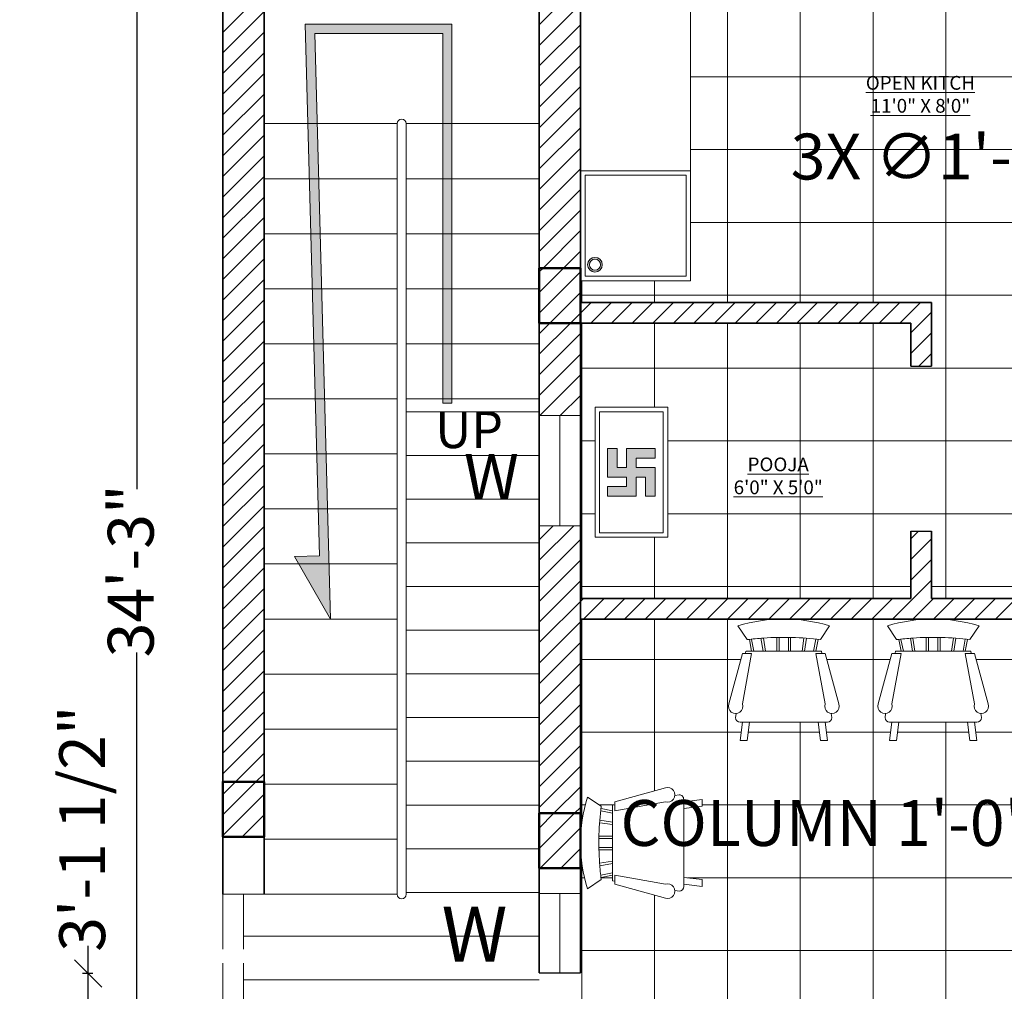
# Model space of a CAD drawing. Units: inches. Extents: x 2036 to 2670, y 319 to 920.
# Tile 3 of 15: x 2036 to 2251, y 579 to 790. Entities that reach past the tile are written whole.
import ezdxf

# ---------------------------------------------------------------- set-up
doc = ezdxf.new("R2010")
doc.units = ezdxf.units.IN
doc.linetypes.add('ACAD_ISO02W100', pattern=[15, 12, -3])
for name, color, linetype, lineweight in [('A-ANNO-DIMS', 2, 'Continuous', 18), ('A-ANNO-SYMB', 7, 'Continuous', 18), ('A-ANNO-SYMB-PATT', 7, 'Continuous', 13), ('A-ANNO-TEXT', 7, 'Continuous', 18), ('A-AREA-IDEN', 7, 'Continuous', 18), ('A-CASE', 7, 'Continuous', 18), ('A-CASE-PATT', 9, 'Continuous', 13), ('A-COLS', 7, 'Continuous', 50), ('A-DOOR', 3, 'Continuous', 25), ('A-FLOR-FIXT', 8, 'Continuous', 18), ('A-FLOR-FIXT-PATT', 8, 'Continuous', 9), ('A-FLOR-OVHD', 1, 'ACAD_ISO02W100', 13), ('A-FLOR-PATT', 8, 'Continuous', 9), ('A-FLOR-STRS', 7, 'Continuous', 18), ('A-FURN', 8, 'Continuous', 18), ('A-GLAZ', 4, 'Continuous', 18), ('A-WALL', 7, 'Continuous', 35)]:
    doc.layers.add(name, color=color, linetype=linetype, lineweight=lineweight)
doc.layers.add('A-COLS-PATT', color=240, linetype='Continuous', lineweight=13, true_color=0xed1f24)
doc.layers.add('A-WALL-PATT', color=52, linetype='Continuous', lineweight=13, true_color=0xc8c92d)
doc.styles.get("Standard").update_dxf_attribs({"font": 'arial.ttf'})
doc.dimstyles.new('ISO-25', dxfattribs={"dimtxt": 10, "dimasz": 6, "dimexe": 1.25, "dimexo": 0.625, "dimtad": 0, "dimdec": 1, "dimlunit": 3, "dimtxsty": 'Standard', "dimblk": 'OBLIQUE', "dimcen": 2.5, "dimclrd": 94, "dimclre": 94, "dimclrt": 1, "dimadec": 0, "dimazin": 0, "dimtfac": 1, "dimtdec": 1, "dimtmove": 0, "dimatfit": 3, "dimfxl": 1, "dimfxlon": 1, "dimarcsym": 0})

# ---------------------------------------------------------------- blocks, each defined once
blk = doc.blocks.new('Chair - Rocking')
for p, q in [((-8, -4.5), (-10, -1.5)), ((8, -4.5), (10, -1.5)), ((-4.5, -7), (-4.96674, -4.19951)), ((-4, -7), (-4.40532, -4.16272)), ((-1.5, -4.05012), (-1.5, -7)), ((-1, -7), (-1, -4.05012)), ((1, -7), (1, -4.04655)), ((1.5, -4.05012), (1.5, -7)), ((4, -7), (4.40187, -4.18694)), ((4.5, -7), (4.96761, -4.19437)), ((-7.5, -4.5), (-7, -7)), ((-6.5, -7), (-7.02225, -4.43)), ((6.5, -7), (7, -4.4057)), ((7.5, -4.5), (7, -7)), ((-9, -7.5), (-12, -18.49999)), ((-7, -7.5), (-9, -7.5)), ((-9, -18.49999), (-7, -7.5)), ((-8.23428, -6.99939), (-8.3093, -7.47958)), ((-8.23041, -7), (8.23915, -7)), ((7, -7.5), (9, -7.5)), ((9, -18.49999), (7, -7.5)), ((8.31071, -7.48854), (8.23449, -7.00073)), ((9, -7.5), (12, -18.49999)), ((-10.36644, -20.64523), (-10.5, -21.49999)), ((10.5, -21.49999), (10.3575, -20.58798)), ((-9, -22.49999), (-9.5, -26.49999)), ((0, -22.49999), (-9.5, -22.49999)), ((-8, -26.49999), (-7.5, -22.49999)), ((0, -22.49999), (9.5, -22.49999)), ((8, -26.49999), (7.5, -22.49999)), ((9, -22.49999), (9.5, -26.49999)), ((-9.5, -26.49999), (-8, -26.49999)), ((9.5, -26.49999), (8, -26.49999))]:
    blk.add_line(p, q)
for centre, radius, start, end in [((0, -34.08333), 34.08333, 72.93847, 107.0615), ((0, -68.25004), 64.25, 93.92211, 97.15267), ((0, -68.25004), 64.25, 82.84733, 93.92211), ((-10.5, -18.99999), 1.58114, 161.5651, 18.43495), ((10.5, -18.99999), 1.58114, 161.5651, 18.43495), ((-9.5, -21.49999), 1, 180, 270), ((9.5, -21.49999), 1, 270, 0)]:
    blk.add_arc(centre, radius, start, end)
blk = doc.blocks.new('_Oblique')
at = {"color": 0, "linetype": 'ByBlock', "lineweight": -2}
blk.add_line((-0.5, -0.5), (0.5, 0.5), dxfattribs=at)
blk = doc.blocks.new('*D13')
at = {"layer": 'A-ANNO-DIMS', "color": 0, "lineweight": -2, "transparency": 16777216}
for p, q in [((2062.98, 875.68), (2060.73, 875.68)), ((2061.98, 875.68), (2061.98, 687.98)), ((2061.98, 464.68), (2061.98, 652.39)), ((2062.98, 464.68), (2060.73, 464.68))]:
    blk.add_line(p, q, dxfattribs=at)
at = {"layer": 'Defpoints', "color": 0, "transparency": 16777216}
for p in [(2080.74, 875.68), (2061.98, 464.68), (2080.74, 464.68)]:
    blk.add_point(p, dxfattribs=at)
at = {"layer": 'A-ANNO-DIMS', "color": 0, "lineweight": -2, "transparency": 16777216, "xscale": 6, "yscale": 6, "zscale": 6}
for p, rotation in [((2061.98, 875.68), 90), ((2061.98, 464.68), 270)]:
    blk.add_blockref('_Oblique', p, dxfattribs=dict(at, rotation=rotation))
at = {"layer": 'A-ANNO-DIMS', "color": 0, "transparency": 16777216, "insert": (2061.98, 670.18), "char_height": 10, "attachment_point": 5, "rotation": 90}
blk.add_mtext('34\'-3"', dxfattribs=at)
blk = doc.blocks.new('COL-9x12')
blk.add_lwpolyline([(9, 0), (0, 0), (0, 12), (9, 12)], close=True)
blk = doc.blocks.new('GLAZ-24x9-PLAN')
for p, q in [((9, 24), (0, 24)), ((4.5, 24), (4.5, 0)), ((9, 0), (0, 0))]:
    blk.add_line(p, q)
blk = doc.blocks.new('*D21')
at = {"layer": 'A-ANNO-DIMS', "color": 94, "lineweight": -2, "transparency": 16777216}
for p, q in [((2297.27, 612.92), (2297.27, 615.17)), ((2309.27, 612.92), (2309.27, 615.17)), ((2297.27, 613.92), (2291.27, 613.92)), ((2309.27, 613.92), (2297.27, 613.92))]:
    blk.add_line(p, q, dxfattribs=at)
at = {"layer": 'Defpoints', "color": 0, "transparency": 16777216}
for p in [(2297.27, 613.92), (2297.27, 612.12), (2309.27, 612.12)]:
    blk.add_point(p, dxfattribs=at)
at = {"layer": 'A-ANNO-DIMS', "color": 94, "lineweight": -2, "transparency": 16777216, "xscale": 6, "yscale": 6, "zscale": 6}
for p, rotation in [((2297.27, 613.92), 179.9999999999962), ((2309.27, 613.92), 359.9999999999962)]:
    blk.add_blockref('_Oblique', p, dxfattribs=dict(at, rotation=rotation))
at = {"layer": 'A-ANNO-DIMS', "color": 1, "transparency": 16777216, "insert": (2228.01, 613.92), "char_height": 10, "attachment_point": 5}
blk.add_mtext('COLUMN 1\'-0" TYP.', dxfattribs=at)
blk = doc.blocks.new('*D54')
at = {"layer": 'A-ANNO-DIMS', "color": 94, "lineweight": -2, "transparency": 16777216}
for p, q in [((2642.09, 545.51), (2642.09, 551.51)), ((2641.09, 545.51), (2643.34, 545.51)), ((2642.09, 513.19), (2642.09, 545.51)), ((2641.09, 513.19), (2643.34, 513.19))]:
    blk.add_line(p, q, dxfattribs=at)
at = {"layer": 'Defpoints', "color": 0, "transparency": 16777216}
for p in [(2158.74, 545.51), (2642.09, 545.51), (2158.74, 513.19)]:
    blk.add_point(p, dxfattribs=at)
at = {"layer": 'A-ANNO-DIMS', "color": 94, "lineweight": -2, "transparency": 16777216, "xscale": 6, "yscale": 6, "zscale": 6}
for p, rotation in [((2642.09, 545.51), 90), ((2642.09, 513.19), 270)]:
    blk.add_blockref('_Oblique', p, dxfattribs=dict(at, rotation=rotation))
at = {"layer": 'A-ANNO-DIMS', "color": 1, "transparency": 16777216, "insert": (2642.09, 577.16), "char_height": 10, "attachment_point": 5, "rotation": 90}
blk.add_mtext('2\'-8 1/2"', dxfattribs=at)
blk = doc.blocks.new('*D55')
at = {"layer": 'A-ANNO-DIMS', "color": 94, "lineweight": -2, "transparency": 16777216}
for p, q in [((2641.09, 582.53), (2643.34, 582.53)), ((2642.09, 582.53), (2642.09, 577.94)), ((2642.09, 545.51), (2642.09, 550.11)), ((2641.09, 545.51), (2643.34, 545.51))]:
    blk.add_line(p, q, dxfattribs=at)
at = {"layer": 'Defpoints', "color": 0, "transparency": 16777216}
for p in [(2158.74, 582.53), (2642.09, 582.53), (2158.74, 545.51)]:
    blk.add_point(p, dxfattribs=at)
at = {"layer": 'A-ANNO-DIMS', "color": 94, "lineweight": -2, "transparency": 16777216, "xscale": 6, "yscale": 6, "zscale": 6}
for p, rotation in [((2642.09, 582.53), 90), ((2642.09, 545.51), 270)]:
    blk.add_blockref('_Oblique', p, dxfattribs=dict(at, rotation=rotation))
at = {"layer": 'A-ANNO-DIMS', "color": 1, "transparency": 16777216, "insert": (2642.09, 564.02), "char_height": 10, "attachment_point": 5, "rotation": 90}
blk.add_mtext('3\'-1"', dxfattribs=at)
blk = doc.blocks.new('*D56')
at = {"layer": 'A-ANNO-DIMS', "color": 94, "lineweight": -2, "transparency": 16777216}
for p, q in [((2642.09, 599.85), (2642.09, 605.85)), ((2641.09, 599.85), (2643.34, 599.85)), ((2642.09, 582.53), (2642.09, 599.85)), ((2641.09, 582.53), (2643.34, 582.53))]:
    blk.add_line(p, q, dxfattribs=at)
at = {"layer": 'Defpoints', "color": 0, "transparency": 16777216}
for p in [(2158.74, 599.85), (2642.09, 599.85), (2158.74, 582.53)]:
    blk.add_point(p, dxfattribs=at)
at = {"layer": 'A-ANNO-DIMS', "color": 94, "lineweight": -2, "transparency": 16777216, "xscale": 6, "yscale": 6, "zscale": 6}
for p, rotation in [((2642.09, 599.85), 90), ((2642.09, 582.53), 270)]:
    blk.add_blockref('_Oblique', p, dxfattribs=dict(at, rotation=rotation))
at = {"layer": 'A-ANNO-DIMS', "color": 1, "transparency": 16777216, "insert": (2642.09, 630.95), "char_height": 10, "attachment_point": 5, "rotation": 90}
blk.add_mtext('1\'-5 1/2"', dxfattribs=at)
blk = doc.blocks.new('*D58')
at = {"layer": 'A-ANNO-DIMS', "color": 94, "lineweight": -2, "transparency": 16777216}
for p, q in [((2224.74, 436.33), (2224.74, 434.08)), ((2270.11, 436.33), (2270.11, 434.08)), ((2224.74, 435.33), (2270.11, 435.33)), ((2270.11, 435.33), (2276.11, 435.33))]:
    blk.add_line(p, q, dxfattribs=at)
at = {"layer": 'Defpoints', "color": 0, "transparency": 16777216}
for p in [(2224.74, 824.68), (2270.11, 824.68), (2270.11, 435.33)]:
    blk.add_point(p, dxfattribs=at)
at = {"layer": 'A-ANNO-DIMS', "color": 94, "lineweight": -2, "transparency": 16777216, "xscale": 6, "yscale": 6, "zscale": 6, "rotation": 180}
blk.add_blockref('_Oblique', (2224.74, 435.33), dxfattribs=at)
at = {"layer": 'A-ANNO-DIMS', "color": 94, "lineweight": -2, "transparency": 16777216, "xscale": 6, "yscale": 6, "zscale": 6}
blk.add_blockref('_Oblique', (2270.11, 435.33), dxfattribs=at)
at = {"layer": 'A-ANNO-DIMS', "color": 1, "transparency": 16777216, "insert": (2301.68, 435.33), "char_height": 10, "attachment_point": 5}
blk.add_mtext('3\'-9 1/2"', dxfattribs=at)
blk = doc.blocks.new('*D59')
at = {"layer": 'A-ANNO-DIMS', "color": 94, "lineweight": -2, "transparency": 16777216}
for p, q in [((2641.09, 714.81), (2643.34, 714.81)), ((2642.09, 714.81), (2642.09, 710.72)), ((2642.09, 678.81), (2642.09, 682.89)), ((2641.09, 678.81), (2643.34, 678.81))]:
    blk.add_line(p, q, dxfattribs=at)
at = {"layer": 'Defpoints', "color": 0, "transparency": 16777216}
for p in [(2235.24, 714.81), (2642.09, 714.81), (2235.24, 678.81)]:
    blk.add_point(p, dxfattribs=at)
at = {"layer": 'A-ANNO-DIMS', "color": 94, "lineweight": -2, "transparency": 16777216, "xscale": 6, "yscale": 6, "zscale": 6}
for p, rotation in [((2642.09, 714.81), 90), ((2642.09, 678.81), 270)]:
    blk.add_blockref('_Oblique', p, dxfattribs=dict(at, rotation=rotation))
at = {"layer": 'A-ANNO-DIMS', "color": 1, "transparency": 16777216, "insert": (2642.09, 696.81), "char_height": 10, "attachment_point": 5, "rotation": 90}
blk.add_mtext('3\'-0"', dxfattribs=at)
blk = doc.blocks.new('*D60')
at = {"layer": 'A-ANNO-DIMS', "color": 94, "lineweight": -2, "transparency": 16777216}
for p, q in [((2051.39, 582.41), (2051.39, 588.41)), ((2052.39, 582.41), (2050.14, 582.41)), ((2051.39, 545.09), (2051.39, 582.41)), ((2052.39, 545.09), (2050.14, 545.09))]:
    blk.add_line(p, q, dxfattribs=at)
at = {"layer": 'Defpoints', "color": 0, "transparency": 16777216}
for p in [(2051.39, 582.41), (2515.24, 582.41), (2515.24, 545.09)]:
    blk.add_point(p, dxfattribs=at)
at = {"layer": 'A-ANNO-DIMS', "color": 94, "lineweight": -2, "transparency": 16777216, "xscale": 6, "yscale": 6, "zscale": 6}
for p, rotation in [((2051.39, 582.41), 90), ((2051.39, 545.09), 270)]:
    blk.add_blockref('_Oblique', p, dxfattribs=dict(at, rotation=rotation))
at = {"layer": 'A-ANNO-DIMS', "color": 1, "transparency": 16777216, "insert": (2051.39, 613.98), "char_height": 10, "attachment_point": 5, "rotation": 90}
blk.add_mtext('3\'-1 1/2"', dxfattribs=at)
blk = doc.blocks.new('*D62')
at = {"layer": 'A-ANNO-DIMS', "color": 94, "lineweight": -2, "transparency": 16777216}
for p in [(2288.93, 759.21), (2317.52, 759.21)]:
    blk.add_line(p, (2300.93, 759.21), dxfattribs=at)
at = {"layer": 'Defpoints', "color": 0, "transparency": 16777216}
for p in [(2300.93, 759.21), (2317.52, 759.21)]:
    blk.add_point(p, dxfattribs=at)
at = {"layer": 'A-ANNO-DIMS', "color": 94, "lineweight": -2, "transparency": 16777216, "xscale": 6, "yscale": 6, "zscale": 6}
for p, rotation in [((2300.93, 759.21), 0.0016372222120452), ((2317.52, 759.21), 180.001637222212)]:
    blk.add_blockref('_Oblique', p, dxfattribs=dict(at, rotation=rotation))
at = {"layer": 'A-ANNO-DIMS', "color": 1, "transparency": 16777216, "insert": (2247.45, 759.21), "char_height": 10, "attachment_point": 5, "rotation": 0.0016}
blk.add_mtext('3X ∅1\'-4 1/2"', dxfattribs=at)

msp = doc.modelspace()

# ---------------------------------------------------------------- hatches: boundary and pattern name
at = {"layer": 'A-ANNO-SYMB-PATT'}
h = msp.add_hatch(color=256, dxfattribs=at)
h.dxf.hatch_style = 1
h.paths.add_polyline_path([(2128.7, 787.34), (2128.7, 706.72), (2130.7, 706.72), (2130.7, 789.34), (2098.74, 789.34), (2101.86, 673.45), (2096.37, 673.3), (2104.24, 659.68), (2100.8, 787.34)])
at = {"layer": 'A-CASE-PATT'}
h = msp.add_hatch(color=256, dxfattribs=at)
h.dxf.hatch_style = 1
h.paths.add_polyline_path([(2175.01, 692.71), (2170.86, 692.71), (2170.86, 694.78), (2175.01, 694.78), (2175.01, 696.85), (2168.78, 696.85), (2168.78, 692.71), (2166.71, 692.71), (2166.71, 696.85), (2164.63, 696.85), (2164.63, 690.63), (2168.78, 690.63), (2168.78, 688.56), (2166.71, 688.56), (2164.63, 688.56), (2164.63, 686.48), (2170.86, 686.48), (2170.86, 690.63), (2172.93, 690.63), (2172.93, 686.48), (2175.01, 686.48)])
at = {"layer": 'A-COLS-PATT'}
h = msp.add_hatch(dxfattribs=at)
h.set_pattern_fill('ANSI31', color=256)
h.paths.add_polyline_path([(2089.74, 875.68), (2080.74, 875.68), (2080.74, 863.68), (2089.74, 863.68)])
h.paths.add_polyline_path([(2089.74, 821.68), (2080.74, 821.68), (2080.74, 809.68), (2089.74, 809.68)])
h.paths.add_polyline_path([(2089.74, 624.2), (2080.74, 624.2), (2080.74, 612.2), (2089.74, 612.2)])
h.paths.add_polyline_path([(2158.74, 506.68), (2149.74, 506.68), (2149.74, 494.68), (2158.74, 494.68)])
h.paths.add_polyline_path([(2158.74, 617.33), (2149.74, 617.33), (2149.74, 605.33), (2158.74, 605.33)])
h.paths.add_polyline_path([(2158.74, 736.18), (2149.74, 736.18), (2149.74, 724.18), (2158.74, 724.18)])
h.paths.add_polyline_path([(2158.74, 852.81), (2149.74, 852.81), (2149.74, 843.81), (2158.74, 843.81)])
h.paths.add_polyline_path([(2161.74, 852.81), (2158.74, 852.81), (2158.74, 843.81), (2161.74, 843.81)])
h.paths.add_polyline_path([(2295.21, 857.66), (2290.74, 857.66), (2290.74, 848.68), (2295.21, 848.68)])
h.paths.add_polyline_path([(2290.74, 857.66), (2283.21, 857.66), (2283.21, 848.66), (2290.74, 848.66)])
h.paths.add_polyline_path([(2443.62, 857.68), (2431.62, 857.68), (2431.62, 848.68), (2443.62, 848.68)])
h.paths.add_polyline_path([(2561.81, 857.68), (2549.81, 857.68), (2549.81, 848.68), (2561.81, 848.68)])
h.paths.add_polyline_path([(2295.24, 737.65), (2290.74, 737.65), (2290.74, 728.68), (2295.24, 728.68)])
h.paths.add_polyline_path([(2309.27, 612.12), (2297.27, 612.12), (2297.27, 603.12), (2309.27, 603.12)])
h.paths.add_polyline_path([(2282.24, 503.68), (2270.24, 503.68), (2270.24, 494.68), (2282.24, 494.68)])
h.paths.add_polyline_path([(2431.74, 746.09), (2427.24, 746.09), (2427.24, 737.09), (2431.74, 737.09)])
h.paths.add_polyline_path([(2439.24, 746.09), (2431.74, 746.09), (2431.74, 737.09), (2439.24, 737.09)])
h.paths.add_polyline_path([(2596.59, 736.59), (2584.59, 736.59), (2584.59, 727.59), (2596.59, 727.59)])
h.paths.add_polyline_path([(2586.39, 623.71), (2574.39, 623.71), (2574.39, 619.18), (2586.39, 619.18)])
h.paths.add_polyline_path([(2586.39, 619.18), (2574.39, 619.18), (2574.39, 614.71), (2586.39, 614.71)])
h.paths.add_polyline_path([(2438.74, 623.68), (2431.24, 623.68), (2431.24, 619.18), (2438.74, 619.18)])
h.paths.add_polyline_path([(2438.74, 619.18), (2431.24, 619.18), (2431.24, 614.68), (2438.74, 614.68)])
h.paths.add_polyline_path([(2431.24, 623.68), (2426.74, 623.68), (2426.74, 614.68), (2431.24, 614.68), (2431.24, 619.18)])
h.paths.add_polyline_path([(2527.24, 503.68), (2515.24, 503.68), (2515.24, 494.68), (2527.24, 494.68)])
h.paths.add_polyline_path([(2590.31, 503.68), (2578.31, 503.68), (2578.31, 494.68), (2590.31, 494.68)])
at = {"layer": 'A-FLOR-FIXT-PATT'}
h = msp.add_hatch(color=256, dxfattribs=at)
h.dxf.hatch_style = 1
h.paths.add_polyline_path([(2160.29, 736.93, 1), (2163.49, 736.93, 1)])
h.paths.add_polyline_path([(2163.11, 736.93, -1), (2160.67, 736.93, -1)], flags=16)
at = {"layer": 'A-FLOR-PATT'}
h = msp.add_hatch(dxfattribs=at)
h.set_pattern_fill('ANSI31', color=256, scale=5, angle=135)
h.paths.add_polyline_path([(2290.74, 659.68), (2158.74, 659.68), (2158.74, 582.53), (2158.74, 545.51), (2158.74, 503.68), (2426.74, 503.68), (2426.74, 614.68), (2426.74, 623.68), (2426.74, 628.18), (2431.24, 628.18), (2431.24, 623.68), (2438.74, 623.68), (2438.74, 619.18), (2574.39, 619.18), (2574.39, 623.71), (2586.39, 623.71), (2586.39, 619.18), (2603.74, 619.18), (2603.74, 824.68), (2431.74, 824.68), (2431.74, 746.09), (2439.24, 746.09), (2439.24, 737.09), (2431.74, 737.09), (2431.74, 659.68), (2427.24, 659.68), (2427.24, 739.48), (2383.24, 739.48), (2383.24, 804.68), (2339.24, 804.68), (2339.24, 749.08), (2295.24, 749.08), (2295.24, 737.65), (2295.27, 737.65), (2295.27, 728.65), (2295.21, 728.65, -0.586418), (2272.74, 728.68), (2272.74, 824.68), (2270.11, 824.68), (2270.11, 829.18), (2290.74, 829.18), (2290.74, 848.66), (2283.21, 848.66), (2283.21, 857.66), (2289.74, 857.66), (2289.74, 874.68), (2158.74, 874.68), (2158.74, 852.81), (2161.74, 852.81), (2161.74, 843.81), (2158.74, 843.81), (2158.74, 829.18), (2224.74, 829.18), (2224.74, 800.68), (2182.74, 800.68), (2182.74, 733.41), (2158.74, 733.41), (2158.74, 728.68), (2235.24, 728.68), (2235.24, 714.81), (2230.74, 714.81), (2230.74, 724.18), (2158.74, 724.18), (2158.74, 664.18), (2230.74, 664.18), (2230.74, 678.81), (2235.24, 678.81), (2235.24, 664.18), (2290.74, 664.18)])
h.paths.add_polyline_path([(2309.27, 612.12), (2309.27, 603.12), (2297.27, 603.12), (2297.27, 612.12)], flags=16)
h.paths.add_polyline_path([(2280.12, 639.11), (2280.26, 638.18, -0.414214), (2279.26, 637.18), (2278.76, 637.18), (2279.26, 633.18), (2277.76, 633.18), (2277.26, 637.18), (2269.76, 637.18), (2262.26, 637.18), (2261.76, 633.18), (2260.26, 633.18), (2260.76, 637.18), (2260.26, 637.18, -0.414214), (2259.26, 638.18), (2259.41, 639.11, -0.541164), (2257.76, 641.18), (2260.76, 652.18), (2261.45, 652.18), (2261.53, 652.68), (2262.76, 652.68), (2262.25, 655.24, 0.001913), (2261.76, 655.18), (2259.76, 658.18, -0.15), (2279.76, 658.18), (2277.76, 655.18, 0.001913), (2277.27, 655.24), (2276.76, 652.68), (2278, 652.68), (2278.07, 652.18), (2278.76, 652.18), (2281.76, 641.18, -0.541163)], flags=16)
h.paths.add_polyline_path([(2245.98, 639.11), (2246.13, 638.18, -0.414214), (2245.13, 637.18), (2244.63, 637.18), (2245.13, 633.18), (2243.63, 633.18), (2243.13, 637.18), (2235.63, 637.18), (2228.13, 637.18), (2227.63, 633.18), (2226.13, 633.18), (2226.63, 637.18), (2226.13, 637.18, -0.414214), (2225.13, 638.18), (2225.27, 639.11, -0.541164), (2223.63, 641.18), (2226.63, 652.18), (2227.32, 652.18), (2227.39, 652.68), (2228.63, 652.68), (2228.12, 655.24, 0.001913), (2227.63, 655.18), (2225.63, 658.18, -0.15), (2245.63, 658.18), (2243.63, 655.18, 0.001913), (2243.14, 655.24), (2242.63, 652.68), (2243.86, 652.68), (2243.94, 652.18), (2244.63, 652.18), (2247.63, 641.18, -0.541163)], flags=16)
h.paths.add_polyline_path([(2351.59, 515.15, -0.151948), (2279.59, 515.15), (2279.59, 537.68), (2273.59, 537.68), (2273.59, 511.68, 0.190476), (2357.59, 511.68), (2357.59, 537.68), (2351.59, 537.68)])
h.paths.add_polyline_path([(2327.59, 536.13), (2327.59, 517.07), (2303.59, 517.07), (2303.59, 536.13)], flags=16)
h.paths.add_polyline_path([(2213.4, 639.11), (2213.55, 638.18, -0.414214), (2212.55, 637.18), (2212.05, 637.18), (2212.55, 633.18), (2211.05, 633.18), (2210.55, 637.18), (2203.05, 637.18), (2195.55, 637.18), (2195.05, 633.18), (2193.55, 633.18), (2194.05, 637.18), (2193.55, 637.18, -0.414214), (2192.55, 638.18), (2192.69, 639.11, -0.541164), (2191.05, 641.18), (2194.05, 652.18), (2194.73, 652.18), (2194.81, 652.68), (2196.05, 652.68), (2195.53, 655.24, 0.001913), (2195.05, 655.18), (2193.05, 658.18, -0.15), (2213.05, 658.18), (2211.05, 655.18, 0.001913), (2210.56, 655.24), (2210.05, 652.68), (2211.28, 652.68), (2211.36, 652.18), (2212.05, 652.18), (2215.05, 641.18, -0.541163)], flags=16)
h.paths.add_polyline_path([(2368.58, 538.02), (2370.52, 538.02), (2371.17, 532.84), (2380.89, 532.84), (2390.6, 532.84), (2391.25, 538.02), (2393.2, 538.02), (2392.55, 532.84), (2380.89, 532.84), (2368.58, 532.84, 0.414214), (2367.28, 531.54), (2367.47, 530.34, -0.483352), (2369.23, 527.65), (2371.82, 513.4), (2370.12, 513.4), (2370.22, 512.75), (2391.56, 512.75), (2391.66, 513.4), (2389.96, 513.4), (2392.55, 527.65, -1.387427), (2396.43, 527.65), (2392.55, 513.4), (2391.66, 513.4), (2391.56, 512.75), (2389.31, 512.75), (2390, 509.37, 0.003796), (2391.25, 509.51), (2393.84, 505.63, -0.15), (2367.93, 505.63), (2370.52, 509.51, 0.003901), (2371.81, 509.36), (2372.47, 512.75), (2370.22, 512.75), (2370.12, 513.4), (2369.23, 513.4), (2365.34, 527.65, -0.541163), (2367.47, 530.34), (2367.28, 531.54, -0.414214), (2368.58, 532.84), (2369.23, 532.84)])
h.paths.add_polyline_path([(2266.74, 538.02), (2266.09, 532.84), (2254.43, 532.84), (2242.12, 532.84, 0.414214), (2240.83, 531.54), (2241.01, 530.34, -0.483352), (2242.77, 527.65), (2245.36, 513.4), (2243.66, 513.4), (2243.76, 512.75), (2265.1, 512.75), (2265.2, 513.4), (2263.5, 513.4), (2266.09, 527.65, -1.387427), (2269.98, 527.65), (2266.09, 513.4), (2265.2, 513.4), (2265.1, 512.75), (2262.85, 512.75), (2263.54, 509.37, 0.003796), (2264.79, 509.51), (2267.39, 505.63, -0.15), (2241.47, 505.63), (2244.07, 509.51, 0.003901), (2245.36, 509.36), (2246.01, 512.75), (2243.76, 512.75), (2243.66, 513.4), (2242.77, 513.4), (2238.88, 527.65, -0.541163), (2241.01, 530.34), (2240.83, 531.54, -0.414214), (2242.12, 532.84), (2242.77, 532.84), (2242.12, 538.02), (2244.07, 538.02), (2244.71, 532.84), (2254.43, 532.84), (2264.15, 532.84), (2264.79, 538.02)])
h.paths.add_polyline_path([(2185.24, 620.36), (2185.24, 618.86), (2181.24, 618.36), (2181.24, 610.86), (2181.24, 603.36), (2185.24, 602.86), (2185.24, 601.36), (2181.24, 601.86), (2181.24, 601.36, -0.414214), (2180.24, 600.36), (2179.31, 600.5, -0.541164), (2177.24, 598.86), (2166.24, 601.86), (2166.24, 602.54), (2165.74, 602.62), (2165.74, 603.86), (2163.18, 603.34, 0.001913), (2163.24, 602.86), (2160.24, 600.86, -0.15), (2160.24, 620.86), (2163.24, 618.86, 0.001913), (2163.18, 618.37), (2165.74, 617.86), (2165.74, 619.09), (2166.24, 619.17), (2166.24, 619.86), (2177.24, 622.86, -0.541163), (2179.31, 621.21), (2180.24, 621.36, -0.414214), (2181.24, 620.36), (2181.24, 619.86)])
h.paths.add_polyline_path([(2470.92, 676.01), (2470.92, 806.13), (2568.52, 806.13), (2568.52, 676.01)], flags=16)
h.paths.add_polyline_path([(2177.74, 677.49), (2161.9, 677.49), (2161.9, 705.85), (2177.74, 705.85)], flags=16)
h.paths.add_polyline_path([(2176.74, 678.49), (2162.9, 678.49), (2162.9, 704.85), (2176.74, 704.85)], flags=0)
h.paths.add_polyline_path([(2175.01, 686.48), (2172.93, 686.48), (2172.93, 690.63), (2170.86, 690.63), (2170.86, 686.48), (2164.63, 686.48), (2164.63, 688.56), (2166.71, 688.56), (2168.78, 688.56), (2168.78, 690.63), (2164.63, 690.63), (2164.63, 696.85), (2166.71, 696.85), (2166.71, 692.71), (2168.78, 692.71), (2168.78, 696.85), (2175.01, 696.85), (2175.01, 694.78), (2170.86, 694.78), (2170.86, 692.71), (2175.01, 692.71)], flags=0)
h.paths.add_polyline_path([(2543.79, 782.71), (2483.94, 782.71), (2483.94, 804.18), (2517.77, 804.18), (2517.77, 782.71), (2521.67, 782.71), (2521.67, 804.18), (2555.5, 804.18), (2555.5, 779.45), (2547.05, 779.45), (2568.52, 757.98), (2543.79, 757.98)], flags=0)
h.paths.add_polyline_path([(2584.59, 727.59), (2584.59, 736.59), (2596.59, 736.59), (2596.59, 727.59)], flags=16)
h.paths.add_polyline_path([(2520.45, 647.03), (2553.79, 647.03), (2553.79, 658.23), (2520.45, 658.23)], flags=24)
h.paths.add_polyline_path([(2299.53, 573.74), (2331.71, 573.74), (2331.71, 584.94), (2299.53, 584.94)], flags=24)
h.paths.add_polyline_path([(2191.59, 685.19), (2212.12, 685.19), (2212.12, 696.38), (2191.59, 696.38)], flags=24)
h.paths.add_polyline_path([(2353.9, 649.86), (2379.08, 649.86), (2379.08, 661.06), (2353.9, 661.06)], flags=24)
h.paths.add_polyline_path([(2214.61, 763.31), (2237.46, 763.31), (2237.46, 779.56), (2214.61, 779.56)], flags=24)
h.paths.add_polyline_path([(2225.09, 819.31), (2269.29, 819.31), (2269.29, 844.04), (2225.09, 844.04)], flags=24)
h.paths.add_polyline_path([(2204.06, 845.04), (2226.92, 845.04), (2226.92, 856.24), (2204.06, 856.24)], flags=24)
h = msp.add_hatch(dxfattribs=at)
h.set_pattern_fill('ANSI31', color=256, scale=5, angle=45)
h.paths.add_polyline_path([(2290.74, 659.68), (2158.74, 659.68), (2158.74, 582.53), (2158.74, 545.51), (2158.74, 503.68), (2426.74, 503.68), (2426.74, 614.68), (2426.74, 623.68), (2426.74, 628.18), (2431.24, 628.18), (2431.24, 623.68), (2438.74, 623.68), (2438.74, 619.18), (2574.39, 619.18), (2574.39, 623.71), (2586.39, 623.71), (2586.39, 619.18), (2603.74, 619.18), (2603.74, 824.68), (2431.74, 824.68), (2431.74, 746.09), (2439.24, 746.09), (2439.24, 737.09), (2431.74, 737.09), (2431.74, 659.68), (2427.24, 659.68), (2427.24, 739.48), (2383.24, 739.48), (2383.24, 804.68), (2339.24, 804.68), (2339.24, 749.08), (2295.24, 749.08), (2295.24, 737.65), (2295.27, 737.65), (2295.27, 728.65), (2295.21, 728.65, -0.586418), (2272.74, 728.68), (2272.74, 824.68), (2270.11, 824.68), (2270.11, 829.18), (2290.74, 829.18), (2290.74, 848.66), (2283.21, 848.66), (2283.21, 857.66), (2289.74, 857.66), (2289.74, 874.68), (2158.74, 874.68), (2158.74, 852.81), (2161.74, 852.81), (2161.74, 843.81), (2158.74, 843.81), (2158.74, 829.18), (2224.74, 829.18), (2224.74, 800.68), (2182.74, 800.68), (2182.74, 733.41), (2158.74, 733.41), (2158.74, 728.68), (2235.24, 728.68), (2235.24, 714.81), (2230.74, 714.81), (2230.74, 724.18), (2158.74, 724.18), (2158.74, 664.18), (2230.74, 664.18), (2230.74, 678.81), (2235.24, 678.81), (2235.24, 664.18), (2290.74, 664.18)])
h.paths.add_polyline_path([(2309.27, 612.12), (2309.27, 603.12), (2297.27, 603.12), (2297.27, 612.12)], flags=16)
h.paths.add_polyline_path([(2280.12, 639.11), (2280.26, 638.18, -0.414214), (2279.26, 637.18), (2278.76, 637.18), (2279.26, 633.18), (2277.76, 633.18), (2277.26, 637.18), (2269.76, 637.18), (2262.26, 637.18), (2261.76, 633.18), (2260.26, 633.18), (2260.76, 637.18), (2260.26, 637.18, -0.414214), (2259.26, 638.18), (2259.41, 639.11, -0.541164), (2257.76, 641.18), (2260.76, 652.18), (2261.45, 652.18), (2261.53, 652.68), (2262.76, 652.68), (2262.25, 655.24, 0.001913), (2261.76, 655.18), (2259.76, 658.18, -0.15), (2279.76, 658.18), (2277.76, 655.18, 0.001913), (2277.27, 655.24), (2276.76, 652.68), (2278, 652.68), (2278.07, 652.18), (2278.76, 652.18), (2281.76, 641.18, -0.541163)], flags=16)
h.paths.add_polyline_path([(2245.98, 639.11), (2246.13, 638.18, -0.414214), (2245.13, 637.18), (2244.63, 637.18), (2245.13, 633.18), (2243.63, 633.18), (2243.13, 637.18), (2235.63, 637.18), (2228.13, 637.18), (2227.63, 633.18), (2226.13, 633.18), (2226.63, 637.18), (2226.13, 637.18, -0.414214), (2225.13, 638.18), (2225.27, 639.11, -0.541164), (2223.63, 641.18), (2226.63, 652.18), (2227.32, 652.18), (2227.39, 652.68), (2228.63, 652.68), (2228.12, 655.24, 0.001913), (2227.63, 655.18), (2225.63, 658.18, -0.15), (2245.63, 658.18), (2243.63, 655.18, 0.001913), (2243.14, 655.24), (2242.63, 652.68), (2243.86, 652.68), (2243.94, 652.18), (2244.63, 652.18), (2247.63, 641.18, -0.541163)], flags=16)
h.paths.add_polyline_path([(2351.59, 537.68), (2351.59, 515.15, -0.151948), (2279.59, 515.15), (2279.59, 537.68), (2273.59, 537.68), (2273.59, 511.68, 0.190476), (2357.59, 511.68), (2357.59, 537.68)])
h.paths.add_polyline_path([(2368.58, 538.02), (2370.52, 538.02), (2371.17, 532.84), (2380.89, 532.84), (2390.6, 532.84), (2391.25, 538.02), (2393.2, 538.02), (2392.55, 532.84), (2380.89, 532.84), (2368.58, 532.84, 0.414214), (2367.28, 531.54), (2367.47, 530.34, -0.483352), (2369.23, 527.65), (2371.82, 513.4), (2370.12, 513.4), (2370.22, 512.75), (2391.56, 512.75), (2391.66, 513.4), (2389.96, 513.4), (2392.55, 527.65, -1.387427), (2396.43, 527.65), (2392.55, 513.4), (2391.66, 513.4), (2391.56, 512.75), (2389.31, 512.75), (2390, 509.37, 0.003796), (2391.25, 509.51), (2393.84, 505.63, -0.15), (2367.93, 505.63), (2370.52, 509.51, 0.003901), (2371.81, 509.36), (2372.47, 512.75), (2370.22, 512.75), (2370.12, 513.4), (2369.23, 513.4), (2365.34, 527.65, -0.541163), (2367.47, 530.34), (2367.28, 531.54, -0.414214), (2368.58, 532.84), (2369.23, 532.84)])
h.paths.add_polyline_path([(2327.59, 536.13), (2327.59, 517.07), (2303.59, 517.07), (2303.59, 536.13)], flags=16)
h.paths.add_polyline_path([(2470.92, 676.01), (2470.92, 806.13), (2568.52, 806.13), (2568.52, 676.01)], flags=16)
h.paths.add_polyline_path([(2266.74, 538.02), (2266.09, 532.84), (2254.43, 532.84), (2242.12, 532.84, 0.414214), (2240.83, 531.54), (2241.01, 530.34, -0.483352), (2242.77, 527.65), (2245.36, 513.4), (2243.66, 513.4), (2243.76, 512.75), (2265.1, 512.75), (2265.2, 513.4), (2263.5, 513.4), (2266.09, 527.65, -1.387427), (2269.98, 527.65), (2266.09, 513.4), (2265.2, 513.4), (2265.1, 512.75), (2262.85, 512.75), (2263.54, 509.37, 0.003796), (2264.79, 509.51), (2267.39, 505.63, -0.15), (2241.47, 505.63), (2244.07, 509.51, 0.003901), (2245.36, 509.36), (2246.01, 512.75), (2243.76, 512.75), (2243.66, 513.4), (2242.77, 513.4), (2238.88, 527.65, -0.541163), (2241.01, 530.34), (2240.83, 531.54, -0.414214), (2242.12, 532.84), (2242.77, 532.84), (2242.12, 538.02), (2244.07, 538.02), (2244.71, 532.84), (2254.43, 532.84), (2264.15, 532.84), (2264.79, 538.02)])
h.paths.add_polyline_path([(2213.4, 639.11), (2213.55, 638.18, -0.414214), (2212.55, 637.18), (2212.05, 637.18), (2212.55, 633.18), (2211.05, 633.18), (2210.55, 637.18), (2203.05, 637.18), (2195.55, 637.18), (2195.05, 633.18), (2193.55, 633.18), (2194.05, 637.18), (2193.55, 637.18, -0.414214), (2192.55, 638.18), (2192.69, 639.11, -0.541164), (2191.05, 641.18), (2194.05, 652.18), (2194.73, 652.18), (2194.81, 652.68), (2196.05, 652.68), (2195.53, 655.24, 0.001913), (2195.05, 655.18), (2193.05, 658.18, -0.15), (2213.05, 658.18), (2211.05, 655.18, 0.001913), (2210.56, 655.24), (2210.05, 652.68), (2211.28, 652.68), (2211.36, 652.18), (2212.05, 652.18), (2215.05, 641.18, -0.541163)], flags=16)
h.paths.add_polyline_path([(2185.24, 620.36), (2185.24, 618.86), (2181.24, 618.36), (2181.24, 610.86), (2181.24, 603.36), (2185.24, 602.86), (2185.24, 601.36), (2181.24, 601.86), (2181.24, 601.36, -0.414214), (2180.24, 600.36), (2179.31, 600.5, -0.541164), (2177.24, 598.86), (2166.24, 601.86), (2166.24, 602.54), (2165.74, 602.62), (2165.74, 603.86), (2163.18, 603.34, 0.001913), (2163.24, 602.86), (2160.24, 600.86, -0.15), (2160.24, 620.86), (2163.24, 618.86, 0.001913), (2163.18, 618.37), (2165.74, 617.86), (2165.74, 619.09), (2166.24, 619.17), (2166.24, 619.86), (2177.24, 622.86, -0.541163), (2179.31, 621.21), (2180.24, 621.36, -0.414214), (2181.24, 620.36), (2181.24, 619.86)])
h.paths.add_polyline_path([(2177.74, 677.49), (2161.9, 677.49), (2161.9, 705.85), (2177.74, 705.85)], flags=16)
h.paths.add_polyline_path([(2176.74, 678.49), (2162.9, 678.49), (2162.9, 704.85), (2176.74, 704.85)], flags=0)
h.paths.add_polyline_path([(2175.01, 686.48), (2172.93, 686.48), (2172.93, 690.63), (2170.86, 690.63), (2170.86, 686.48), (2164.63, 686.48), (2164.63, 688.56), (2166.71, 688.56), (2168.78, 688.56), (2168.78, 690.63), (2164.63, 690.63), (2164.63, 696.85), (2166.71, 696.85), (2166.71, 692.71), (2168.78, 692.71), (2168.78, 696.85), (2175.01, 696.85), (2175.01, 694.78), (2170.86, 694.78), (2170.86, 692.71), (2175.01, 692.71)], flags=0)
h.paths.add_polyline_path([(2543.79, 782.71), (2483.94, 782.71), (2483.94, 804.18), (2517.77, 804.18), (2517.77, 782.71), (2521.67, 782.71), (2521.67, 804.18), (2555.5, 804.18), (2555.5, 779.45), (2547.05, 779.45), (2568.52, 757.98), (2543.79, 757.98)], flags=0)
h.paths.add_polyline_path([(2584.59, 727.59), (2584.59, 736.59), (2596.59, 736.59), (2596.59, 727.59)], flags=16)
h.paths.add_polyline_path([(2520.45, 647.03), (2553.79, 647.03), (2553.79, 658.23), (2520.45, 658.23)], flags=24)
h.paths.add_polyline_path([(2299.53, 573.74), (2331.71, 573.74), (2331.71, 584.94), (2299.53, 584.94)], flags=24)
h.paths.add_polyline_path([(2191.59, 685.19), (2212.12, 685.19), (2212.12, 696.38), (2191.59, 696.38)], flags=24)
h.paths.add_polyline_path([(2353.9, 649.86), (2379.08, 649.86), (2379.08, 661.06), (2353.9, 661.06)], flags=24)
h.paths.add_polyline_path([(2214.61, 763.31), (2237.46, 763.31), (2237.46, 779.56), (2214.61, 779.56)], flags=24)
h.paths.add_polyline_path([(2225.09, 819.31), (2269.29, 819.31), (2269.29, 844.04), (2225.09, 844.04)], flags=24)
h.paths.add_polyline_path([(2204.06, 845.04), (2226.92, 845.04), (2226.92, 856.24), (2204.06, 856.24)], flags=24)
h = msp.add_hatch(dxfattribs=at)
h.set_pattern_fill('ANSI31', color=256, scale=3, angle=135)
h.paths.add_polyline_path([(2149.74, 582.53), (2149.74, 707.68), (2120.74, 707.68), (2120.74, 599.68, -1), (2118.74, 599.68), (2085.24, 599.68), (2085.24, 506.68), (2089.74, 506.68), (2089.74, 494.68), (2085.24, 494.68), (2085.24, 469.18), (2608.24, 469.18), (2608.24, 494.68), (2149.74, 494.68), (2149.74, 506.68), (2149.74, 545.51)])
h.paths.add_polyline_path([(2143.58, 686.71), (2149.03, 686.71), (2149.03, 692.89), (2143.58, 692.89)], flags=24)
h.paths.add_polyline_path([(2125.99, 700.31), (2133.31, 700.31), (2133.31, 706.49), (2125.99, 706.49)], flags=24)
at = {"layer": 'A-WALL-PATT'}
h = msp.add_hatch(dxfattribs=at)
h.set_pattern_fill('ANSI31', color=256)
h.paths.add_polyline_path([(2089.74, 863.68), (2080.74, 863.68), (2080.74, 821.68), (2089.74, 821.68)])
h.paths.add_polyline_path([(2089.74, 809.68), (2080.74, 809.68), (2080.74, 624.2), (2089.74, 624.2), (2089.74, 707.68), (2089.74, 767.68)])
h.paths.add_polyline_path([(2149.74, 818.68), (2089.74, 818.68), (2089.74, 809.68), (2149.74, 809.68)])
h.paths.add_polyline_path([(2158.74, 875.68), (2089.74, 875.68), (2089.74, 866.68), (2149.74, 866.68), (2149.74, 852.81), (2158.74, 852.81)])
h.paths.add_polyline_path([(2158.74, 843.81), (2149.74, 843.81), (2149.74, 736.18), (2158.74, 736.18), (2158.74, 824.68)])
h.paths.add_polyline_path([(2181.31, 829.18), (2158.74, 829.18), (2158.74, 824.68), (2181.31, 824.68)])
h.paths.add_polyline_path([(2224.74, 829.18), (2212.72, 829.18), (2212.72, 824.68), (2224.74, 824.68)])
h.paths.add_polyline_path([(2177.02, 503.68), (2158.74, 503.68), (2158.74, 494.68), (2177.02, 494.68)])
h.paths.add_polyline_path([(2158.74, 664.18), (2158.74, 680.02), (2149.74, 680.02), (2149.74, 617.33), (2158.74, 617.33)])
h.paths.add_polyline_path([(2158.74, 724.18), (2149.74, 724.18), (2149.74, 704.02), (2158.74, 704.02)])
h.paths.add_polyline_path([(2235.24, 728.68), (2158.74, 728.68), (2158.74, 724.18), (2230.74, 724.18), (2230.74, 714.81), (2235.24, 714.81)])
h.paths.add_polyline_path([(2290.74, 664.18), (2235.24, 664.18), (2235.24, 678.81), (2230.74, 678.81), (2230.74, 664.18), (2158.74, 664.18), (2158.74, 659.68), (2290.74, 659.68)])
h.paths.add_polyline_path([(2270.24, 503.68), (2227.17, 503.68), (2227.17, 494.68), (2270.24, 494.68)])
h.paths.add_polyline_path([(2515.24, 503.68), (2380.89, 503.68), (2380.89, 494.68), (2515.24, 494.68)])
h.paths.add_polyline_path([(2292.21, 503.68), (2282.24, 503.68), (2282.24, 494.68), (2292.21, 494.68)])
h.paths.add_polyline_path([(2578.31, 503.68), (2527.24, 503.68), (2527.24, 494.68), (2578.31, 494.68)])
h.paths.add_polyline_path([(2603.74, 503.68), (2590.31, 503.68), (2590.31, 494.68), (2603.74, 494.68)])
h.paths.add_polyline_path([(2612.74, 503.68), (2603.74, 503.68), (2603.74, 494.68), (2612.74, 494.68)])
h.paths.add_polyline_path([(2549.81, 857.68), (2443.62, 857.68), (2443.62, 848.68), (2549.81, 848.68)])
h.paths.add_polyline_path([(2295.24, 848.66), (2290.74, 848.66), (2290.74, 829.18), (2270.11, 829.18), (2270.11, 824.68), (2290.74, 824.68), (2290.74, 737.65), (2295.24, 737.65)])
h.paths.add_polyline_path([(2431.74, 737.09), (2427.24, 737.09), (2427.24, 659.68), (2431.74, 659.68)])
h.paths.add_polyline_path([(2431.74, 848.68), (2427.24, 848.68), (2427.24, 746.09), (2431.74, 746.09)])
h.paths.add_polyline_path([(2574.39, 619.18), (2495.46, 619.18), (2495.46, 614.68), (2574.39, 614.68)])
h.paths.add_polyline_path([(2461.84, 619.18), (2438.74, 619.18), (2438.74, 614.68), (2461.84, 614.68)])
h.paths.add_polyline_path([(2603.74, 619.18), (2586.39, 619.18), (2586.39, 614.68), (2603.74, 614.68)], flags=17)

# ---------------------------------------------------------------- linework, layer by layer
at = {"layer": 'A-ANNO-SYMB'}
for p, q in [((2098.74, 789.34), (2101.86, 673.45)), ((2130.7, 789.34), (2098.74, 789.34)), ((2130.7, 706.72), (2130.7, 789.34)), ((2128.7, 787.34), (2100.8, 787.34)), ((2100.8, 787.34), (2104.24, 659.68)), ((2128.7, 706.72), (2128.7, 787.34)), ((2128.7, 706.72), (2130.7, 706.72)), ((2096.37, 673.3), (2101.86, 673.45)), ((2104.24, 659.68), (2096.37, 673.3))]:
    msp.add_line(p, q, dxfattribs=at)
at = {"layer": 'A-CASE'}
for p, q in [((2182.74, 800.68), (2182.74, 733.41)), ((2182.74, 733.41), (2158.74, 733.41)), ((2164.63, 696.85), (2166.71, 696.85)), ((2164.63, 696.85), (2164.63, 690.63)), ((2166.71, 696.85), (2166.71, 692.71)), ((2168.78, 692.71), (2168.78, 696.85)), ((2170.86, 694.78), (2170.86, 692.71)), ((2166.71, 692.71), (2168.78, 692.71)), ((2175.01, 692.71), (2170.86, 692.71)), ((2175.01, 692.71), (2175.01, 686.48)), ((2168.78, 690.63), (2164.63, 690.63)), ((2168.78, 688.56), (2168.78, 690.63)), ((2172.93, 690.63), (2170.86, 690.63)), ((2170.86, 690.63), (2170.86, 686.48)), ((2172.93, 686.48), (2172.93, 690.63)), ((2164.63, 688.56), (2166.71, 688.56)), ((2164.63, 688.56), (2164.63, 686.48)), ((2166.71, 688.56), (2168.78, 688.56)), ((2170.86, 686.48), (2164.63, 686.48)), ((2175.01, 686.48), (2172.93, 686.48))]:
    msp.add_line(p, q, dxfattribs=at)
for points in [[(2161.9, 705.85), (2177.74, 705.85), (2177.74, 677.49), (2161.9, 677.49)], [(2162.9, 704.85), (2176.74, 704.85), (2176.74, 678.49), (2162.9, 678.49)]]:
    msp.add_lwpolyline(points, close=True, dxfattribs=at)
msp.add_lwpolyline([(2168.78, 696.85), (2175.01, 696.85), (2175.01, 694.78), (2170.86, 694.78)], dxfattribs=at)
at = {"layer": 'A-DOOR'}
for p, q in [((2230.74, 714.81), (2235.24, 714.81)), ((2230.74, 678.81), (2235.24, 678.81)), ((2149.74, 582.53), (2158.74, 582.53))]:
    msp.add_line(p, q, dxfattribs=at)
at = {"layer": 'A-FLOR-FIXT'}
for p, q in [((2182.65, 757.41), (2158.74, 757.41)), ((2181.74, 756.41), (2159.74, 756.41)), ((2159.74, 756.41), (2159.74, 734.41)), ((2181.74, 756.41), (2181.74, 734.41)), ((2181.74, 734.41), (2159.74, 734.41))]:
    msp.add_line(p, q, dxfattribs=at)
for radius in [1.6, 1.22]:
    msp.add_circle((2161.89, 736.93), radius, dxfattribs=at)
at = {"layer": 'A-FLOR-OVHD'}
for p, q in [((2080.74, 599.68), (2080.74, 464.68)), ((2085.24, 599.68), (2085.24, 506.68))]:
    msp.add_line(p, q, dxfattribs=at)
at = {"layer": 'A-FLOR-STRS'}
for p, q in [((2118.74, 767.68), (2089.74, 767.68)), ((2118.74, 767.68), (2118.74, 707.68)), ((2149.74, 767.68), (2120.74, 767.68)), ((2120.74, 767.68), (2120.74, 707.68)), ((2118.74, 755.68), (2089.74, 755.68)), ((2149.74, 755.68), (2120.74, 755.68)), ((2118.74, 743.68), (2089.74, 743.68)), ((2149.74, 743.68), (2120.74, 743.68)), ((2118.74, 731.68), (2089.74, 731.68)), ((2149.74, 731.68), (2120.74, 731.68)), ((2118.74, 719.68), (2089.74, 719.68)), ((2149.74, 719.68), (2120.74, 719.68)), ((2118.74, 707.68), (2089.74, 707.68)), ((2118.74, 599.68), (2118.74, 707.68)), ((2149.74, 707.68), (2120.74, 707.68)), ((2120.74, 707.68), (2120.74, 599.68)), ((2118.74, 695.68), (2089.74, 695.68)), ((2118.74, 683.68), (2089.74, 683.68)), ((2118.74, 671.68), (2089.74, 671.68)), ((2118.74, 659.68), (2089.74, 659.68)), ((2118.74, 647.68), (2089.74, 647.68)), ((2118.74, 635.68), (2089.74, 635.68)), ((2118.74, 623.68), (2089.74, 623.68)), ((2118.74, 611.68), (2089.74, 611.68)), ((2118.74, 599.68), (2080.74, 599.68))]:
    msp.add_line(p, q, dxfattribs=at)
for centre, start, end in [((2119.74, 767.68), 0, 180), ((2119.74, 599.68), 180, 0)]:
    msp.add_arc(centre, 1, start, end, dxfattribs=at)
at = {"layer": 'A-GLAZ'}
for p, q in [((2149.74, 599.85), (2158.74, 599.85)), ((2154.24, 599.85), (2154.24, 582.53))]:
    msp.add_line(p, q, dxfattribs=at)
at = {"layer": 'A-WALL'}
for p, q in [((2080.74, 875.68), (2080.74, 599.68)), ((2089.74, 866.68), (2089.74, 767.68)), ((2149.74, 866.68), (2149.74, 582.53)), ((2158.74, 824.68), (2158.74, 728.68)), ((2089.74, 767.68), (2089.74, 707.68)), ((2158.74, 728.68), (2235.24, 728.68)), ((2158.74, 728.68), (2158.74, 724.18)), ((2235.24, 728.68), (2235.24, 714.81)), ((2158.74, 724.18), (2230.74, 724.18)), ((2158.74, 724.18), (2158.74, 664.18)), ((2230.74, 724.18), (2230.74, 714.81)), ((2089.74, 707.68), (2089.74, 599.68)), ((2230.74, 678.81), (2230.74, 664.18)), ((2235.24, 678.81), (2235.24, 664.18)), ((2158.74, 664.18), (2230.74, 664.18)), ((2158.74, 664.18), (2158.74, 582.53)), ((2235.24, 664.18), (2290.74, 664.18)), ((2158.74, 659.68), (2290.74, 659.68))]:
    msp.add_line(p, q, dxfattribs=at)

# ---------------------------------------------------------------- block references
at = {"layer": 'A-COLS'}
for p in [(2149.73, 724.18), (2080.74, 612.2), (2149.73, 605.33)]:
    msp.add_blockref('COL-9x12', p, dxfattribs=at)
at = {"layer": 'A-FURN'}
for p in [(2203.05, 659.68), (2235.63, 659.68)]:
    msp.add_blockref('Chair - Rocking', p, dxfattribs=at)
at = {"layer": 'A-FURN', "rotation": 89.99999999999999}
msp.add_blockref('Chair - Rocking', (2158.74, 610.86), dxfattribs=at)
at = {"layer": 'A-GLAZ', "rotation": 180}
msp.add_blockref('GLAZ-24x9-PLAN', (2158.74, 704.02), dxfattribs=at)

# ---------------------------------------------------------------- texts
at = {"layer": 'A-ANNO-TEXT', "attachment_point": 1}
for s, width, insert, char_height in [('UP', 7.2943, (2127.06, 704.95), 8), ('W', 27.6972, (2133.33, 695.67), 10), ('W', 27.6972, (2128.44, 597), 12)]:
    msp.add_mtext_dynamic_manual_height_columns(s, width=width, gutter_width=12.5, heights=[0], dxfattribs=dict(at, insert=insert, char_height=char_height))
at = {"layer": 'A-AREA-IDEN', "char_height": 3, "attachment_point": 1}
for s, width, insert in [('\\pxqc;{\\LOPEN KITCH\\P11\'0" X 8\'0"}', 37.4192, (2214.13, 778.07)), ('\\pxqc;{\\LPOOJA \\P6\'0" X 5\'0"}', 24.0713, (2189.8, 694.89))]:
    msp.add_mtext_dynamic_manual_height_columns(s, width=width, gutter_width=12.5, heights=[0], dxfattribs=dict(at, insert=insert))

# ---------------------------------------------------------------- dimensions: what is measured, and where the dimension line sits
at = {"layer": 'A-ANNO-DIMS'}
for base, p1, p2, override, picture, middle in [((2061.98, 464.68), (2080.74, 875.68), (2080.74, 464.68), {"dimclrd": 0, "dimclre": 0, "dimclrt": 0}, '*D13', (2061.98, 670.18)), ((2642.09, 714.81), (2235.24, 678.81), (2235.24, 714.81), {"dimdec": 1, "dimlfac": 1, "dimrnd": 0, "dimzin": 1, "dimdsep": 46, "dimlunit": 4, "dimfrac": 2}, '*D59', (2642.09, 696.81)), ((2642.09, 599.85), (2158.74, 582.53), (2158.74, 599.85), {"dimdec": 1, "dimlfac": 1, "dimrnd": 0, "dimzin": 1, "dimdsep": 46, "dimlunit": 4, "dimfrac": 2}, '*D56', (2642.09, 630.95)), ((2051.39, 582.41), (2515.24, 545.09), (2515.24, 582.41), {"dimdec": 1, "dimlfac": 1, "dimrnd": 0, "dimzin": 1, "dimdsep": 46, "dimlunit": 4, "dimfrac": 2}, '*D60', (2051.39, 613.98)), ((2642.09, 545.51), (2158.74, 513.19), (2158.74, 545.51), {"dimdec": 1, "dimlfac": 1, "dimrnd": 0, "dimzin": 1, "dimdsep": 46, "dimlunit": 4, "dimfrac": 2}, '*D54', (2642.09, 577.16)), ((2642.09, 582.53), (2158.74, 545.51), (2158.74, 582.53), {"dimdec": 1, "dimlfac": 1, "dimrnd": 0, "dimzin": 1, "dimdsep": 46, "dimlunit": 4, "dimfrac": 2}, '*D55', (2642.09, 564.02))]:
    dim = msp.add_linear_dim(base=base, p1=p1, p2=p2, angle=90, dimstyle='ISO-25', override=override, dxfattribs=at)
    dim.commit()
    dim.dimension.update_dxf_attribs({"geometry": picture, "text_midpoint": middle})
dim = msp.add_linear_dim(base=(2270.11, 435.33), p1=(2224.74, 824.68), p2=(2270.11, 824.68), dimstyle='ISO-25', override={"dimdec": 1, "dimlfac": 1, "dimrnd": 0, "dimzin": 1, "dimdsep": 46, "dimlunit": 4, "dimfrac": 2}, dxfattribs=at)
dim.commit()
dim.dimension.update_dxf_attribs({"geometry": '*D58', "text_midpoint": (2301.68, 435.33)})
dim = msp.add_diameter_dim_2p(p1=(2317.52, 759.21), p2=(2300.93, 759.21), text='3X <>', dimstyle='ISO-25', override={"dimdec": 1, "dimlfac": 1, "dimrnd": 0, "dimzin": 1, "dimdsep": 46, "dimlunit": 4, "dimfrac": 2}, dxfattribs=at)
dim.commit()
dim.dimension.update_dxf_attribs({"geometry": '*D62', "text_midpoint": (2247.45, 759.21)})
dim = msp.add_linear_dim(base=(2297.27, 613.92), p1=(2309.27, 612.12), p2=(2297.27, 612.12), angle=180, text='COLUMN <> TYP.', dimstyle='ISO-25', override={"dimdec": 1, "dimlfac": 1, "dimrnd": 0, "dimzin": 1, "dimdsep": 46, "dimlunit": 4, "dimfrac": 2}, dxfattribs=at)
dim.commit()
dim.dimension.update_dxf_attribs({"geometry": '*D21', "text_midpoint": (2228.01, 613.92)})

doc.saveas('drawing.dxf')
